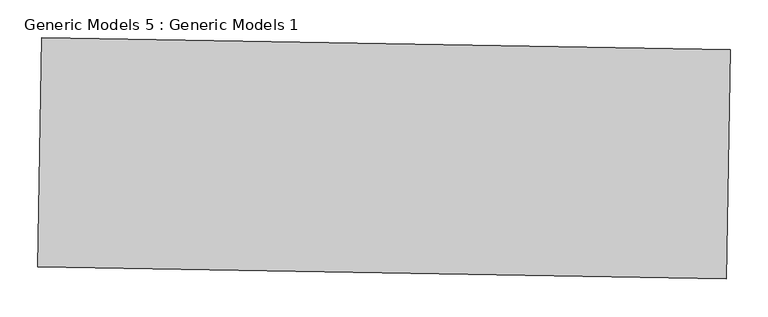
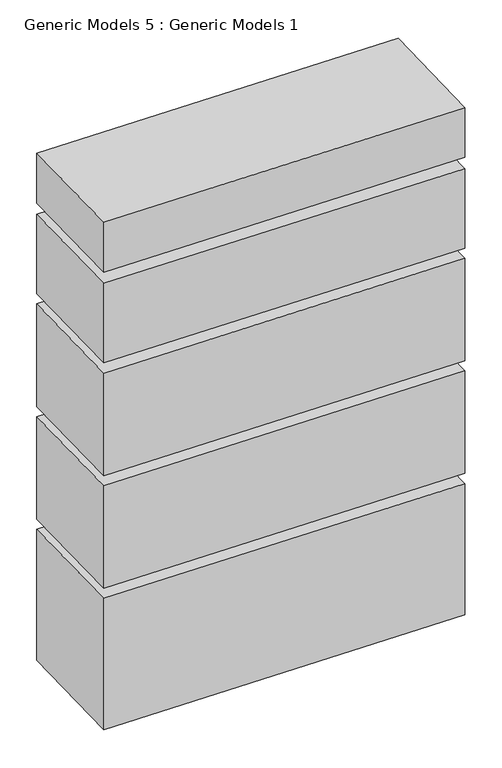
"""IFC4 building model written with IfcOpenShell, lengths in millimetres: proxy geometry, Generic Models 5 : Generic Models 1."""

from ifc_helpers import new_model, si_unit, frame, origin, place, context, project, spatial, polyline, outline, extrude, source, transform, mapped, element, save


def generic_models_5_generic_models_1_3fb950e5(model_context):
    return source(origin(), model_context, "Body", "SweptSolid", [
        extrude(outline(polyline([(2277.5248225, -11509.9433502), (1363.2640901, -11493.9848697), (1368.5835836, -11189.2312922), (2282.844316, -11205.1897727), (2277.5248225, -11509.9433502)])), frame((0.0, 0.0, 1263.5574996), z_axis=(0.0, 0.0, 1.0), x_axis=(1.0, 0.0, 0.0)), (0.0, 0.0, 1.0), 134.9289866),
        extrude(outline(polyline([(2277.5248225, -11509.9433502), (1363.2640901, -11493.9848697), (1368.5835836, -11189.2312922), (2282.844316, -11205.1897727), (2277.5248225, -11509.9433502)])), frame((0.0, 0.0, 26.8864862), z_axis=(0.0, 0.0, 1.0), x_axis=(1.0, 0.0, 0.0)), (0.0, 0.0, 1.0), 354.4191875),
        extrude(outline(polyline([(2277.5248225, -11509.9433502), (1363.2640901, -11493.9848697), (1368.5835836, -11189.2312922), (2282.844316, -11205.1897727), (2277.5248225, -11509.9433502)])), frame((0.0, 0.0, 1018.4973826), z_axis=(0.0, 0.0, 1.0), x_axis=(1.0, 0.0, 0.0)), (0.0, 0.0, 1.0), 214.5718039),
        extrude(outline(polyline([(2277.5248225, -11509.9433502), (1363.2640901, -11493.9848697), (1368.5835836, -11189.2312922), (2282.844316, -11205.1897727), (2277.5248225, -11509.9433502)])), frame((0.0, 0.0, 713.6973826), z_axis=(0.0, 0.0, 1.0), x_axis=(1.0, 0.0, 0.0)), (0.0, 0.0, 1.0), 277.2082911),
        extrude(outline(polyline([(2277.5248225, -11509.9433502), (1363.2640901, -11493.9848697), (1368.5835836, -11189.2312922), (2282.844316, -11205.1897727), (2277.5248225, -11509.9433502)])), frame((0.0, 0.0, 408.8973826), z_axis=(0.0, 0.0, 1.0), x_axis=(1.0, 0.0, 0.0)), (0.0, 0.0, 1.0), 277.2082911),
    ])


if __name__ == "__main__":
    model = new_model("IFC4")
    model_context = context("Model", 3, world=origin())
    ifc_project = project(units=[si_unit("LENGTHUNIT", "METRE", prefix="MILLI")], contexts=[model_context])
    site = spatial("IfcSite", under=ifc_project)
    building = spatial("IfcBuilding", under=site)
    placement = place(None, origin())
    generic_models_5_generic_models_1_shape = generic_models_5_generic_models_1_3fb950e5(model_context)
    element("IfcBuildingElementProxy", 1, Name="Generic Models 5 : Generic Models 1", ObjectType="Generic Models 5 : Generic Models 1", at=placement, inside=building, context=model_context, shape_type="MappedRepresentation", body=[
        mapped(generic_models_5_generic_models_1_shape, transform((0.0, 0.0, 0.0), x_axis=(1.0, 0.0, 0.0), y_axis=(0.0, 1.0, 0.0), z_axis=(0.0, 0.0, 1.0))),
    ])
    save(model, "model.ifc")

# Revit data of these elements
# Element 1 (IfcBuildingElementProxy, "Generic Models 5 : Generic Models 1")
#   Materials on its faces: "Parking Stripe"
# Materials
#   "Parking Stripe": class "Paint", colour RGB 250 250 91, transparency 0, Cost = 0
